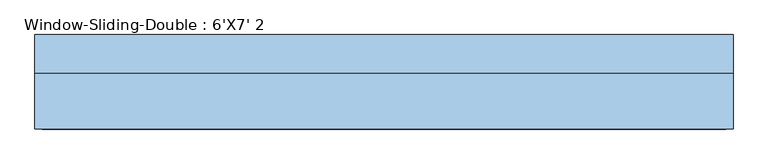
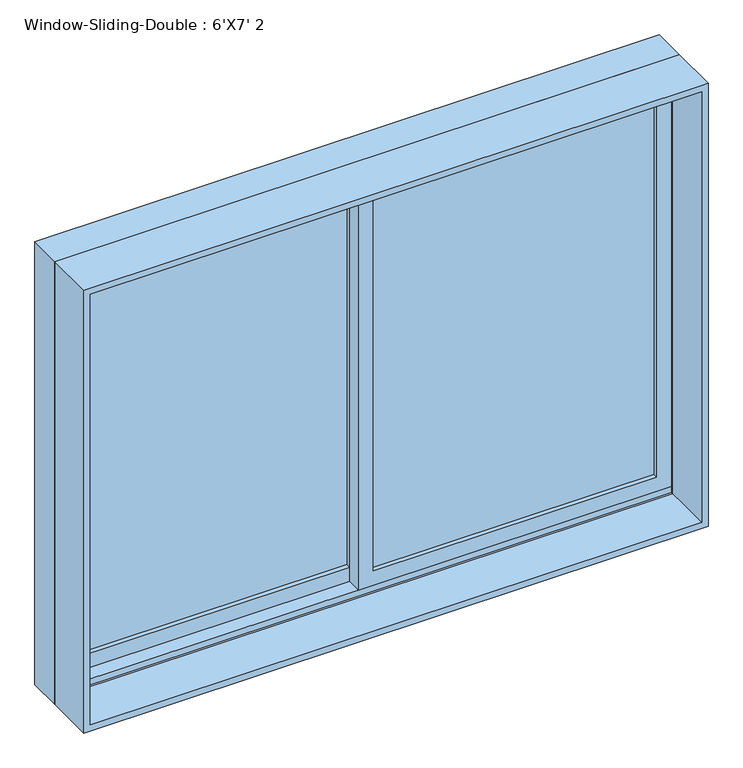
"""IFC4 building model written with IfcOpenShell, lengths in millimetres: window geometry, Window-Sliding-Double : 6'X7' 2."""

from ifc_helpers import new_model, si_unit, frame, origin, place, context, project, spatial, polyline, outline, extrude, faceted_brep, source, transform, mapped, element, save


def window_sliding_double_6_x7_2_7e5eac46(model_context):
    return source(origin(), model_context, "Body", "SolidModel", [
        extrude(outline(polyline([(952.5, 895.35), (2266.95, 895.35), (2266.95, -22.225), (952.5, -22.225), (952.5, 895.35)]), holes=[polyline([(996.95, 22.225), (2222.5, 22.225), (2222.5, 850.9), (996.95, 850.9), (996.95, 22.225)])]), frame((0.0, 34.29, 0.0), z_axis=(0.0, 1.0, 0.0), x_axis=(0.0, 0.0, 1.0)), (0.0, 0.0, 1.0), 44.45),
        extrude(outline(polyline([(933.45, -895.35), (933.45, 22.225), (2266.95, 22.225), (2266.95, -895.35), (933.45, -895.35)]), holes=[polyline([(2222.5, -22.225), (996.95, -22.225), (996.95, -850.9), (2222.5, -850.9), (2222.5, -22.225)])]), frame((0.0, 78.74, 0.0), z_axis=(0.0, 1.0, 0.0), x_axis=(0.0, 0.0, 1.0)), (0.0, 0.0, 1.0), 44.45),
        extrude(outline(polyline([(-22.225, 110.49), (-22.225, 104.14), (-850.9, 104.14), (-850.9, 110.49), (-22.225, 110.49)])), frame((0.0, 0.0, 996.95), z_axis=(0.0, 0.0, 1.0), x_axis=(1.0, 0.0, 0.0)), (0.0, 0.0, 1.0), 1225.55),
        extrude(outline(polyline([(-22.225, 97.79), (-22.225, 91.44), (-850.9, 91.44), (-850.9, 97.79), (-22.225, 97.79)])), frame((0.0, 0.0, 996.95), z_axis=(0.0, 0.0, 1.0), x_axis=(1.0, 0.0, 0.0)), (0.0, 0.0, 1.0), 1225.55),
        extrude(outline(polyline([(850.9, 66.04), (850.9, 59.69), (22.225, 59.69), (22.225, 66.04), (850.9, 66.04)])), frame((0.0, 0.0, 996.95), z_axis=(0.0, 0.0, 1.0), x_axis=(1.0, 0.0, 0.0)), (0.0, 0.0, 1.0), 1225.55),
        extrude(outline(polyline([(850.9, 53.34), (850.9, 46.99), (22.225, 46.99), (22.225, 53.34), (850.9, 53.34)])), frame((0.0, 0.0, 996.95), z_axis=(0.0, 0.0, 1.0), x_axis=(1.0, 0.0, 0.0)), (0.0, 0.0, 1.0), 1225.55),
        extrude(outline(polyline([(2286.0, -914.4), (914.4, -914.4), (914.4, 914.4), (2286.0, 914.4), (2286.0, -914.4)]), holes=[polyline([(2266.95, 895.35), (933.45, 895.35), (933.45, -895.35), (2266.95, -895.35), (2266.95, 895.35)])]), frame((0.0, -118.11, 0.0), z_axis=(0.0, 1.0, 0.0), x_axis=(0.0, 0.0, 1.0)), (0.0, 0.0, 1.0), 146.05),
        faceted_brep([(-914.4, 27.94, 914.4), (-914.4, 129.54, 914.4), (914.4, 129.54, 914.4), (914.4, 27.94, 914.4), (-873.4778905, 129.54, 2245.0778905), (-873.4778905, 123.19, 2245.0778905), (-873.4778905, 123.19, 933.45), (-873.4778905, 129.54, 933.45), (873.4778905, 123.19, 2245.0778905), (873.4778905, 123.19, 933.45), (895.35, 123.19, 933.45), (895.35, 123.19, 2266.95), (-895.35, 123.19, 2266.95), (-895.35, 123.19, 933.45), (-895.35, 27.94, 2266.95), (-895.35, 27.94, 933.45), (-895.35, 34.29, 933.45), (-895.35, 34.29, 952.5), (-895.35, 78.74, 952.5), (-895.35, 78.74, 933.45), (914.4, 27.94, 2286.0), (-914.4, 27.94, 2286.0), (895.35, 27.94, 2266.95), (895.35, 27.94, 933.45), (-914.4, 129.54, 2286.0), (914.4, 129.54, 2286.0), (873.4778905, 129.54, 933.45), (873.4778905, 129.54, 2245.0778905), (895.35, 78.74, 933.45), (895.35, 78.74, 952.5), (895.35, 34.29, 952.5), (895.35, 34.29, 933.45)], [[[0, 1, 2, 3]], [[4, 5, 6, 7]], [[5, 8, 9, 10, 11, 12, 13, 6]], [[12, 14, 15, 16, 17, 18, 19, 13]], [[0, 3, 20, 21], [22, 23, 15, 14]], [[24, 1, 0, 21]], [[2, 1, 24, 25], [4, 7, 26, 27]], [[5, 4, 27, 8]], [[12, 11, 22, 14]], [[21, 20, 25, 24]], [[8, 27, 26, 9]], [[22, 11, 10, 28, 29, 30, 31, 23]], [[20, 3, 2, 25]], [[26, 7, 6, 13, 19, 28, 10, 9]], [[28, 19, 18, 29]], [[29, 18, 17, 30]], [[30, 17, 16, 31]], [[15, 23, 31, 16]]]),
    ])


if __name__ == "__main__":
    model = new_model("IFC4")
    model_context = context("Model", 3, world=origin())
    ifc_project = project(units=[si_unit("LENGTHUNIT", "METRE", prefix="MILLI")], contexts=[model_context])
    site = spatial("IfcSite", under=ifc_project)
    building = spatial("IfcBuilding", under=site)
    placement = place(None, origin())
    window_sliding_double_6_x7_2_shape = window_sliding_double_6_x7_2_7e5eac46(model_context)
    element("IfcWindow", 1, ObjectType="Window-Sliding-Double : 6'X7' 2", at=placement, inside=building, context=model_context, shape_type="MappedRepresentation", body=[
        mapped(window_sliding_double_6_x7_2_shape, transform((0.0, 0.0, 0.0), x_axis=(1.0, 0.0, 0.0), y_axis=(0.0, 1.0, 0.0), z_axis=(0.0, 0.0, 1.0))),
    ])
    save(model, "model.ifc")

# Revit data of these elements
# Type "Window-Sliding-Double : 6'X7' 2"
#   Type Mark = "23"
#   Fire Rating = "0.5h"
#   Assembly Code = "B2020100"
#   Analytic Construction = "Double glazing - domestic"
#   Window Inset [instance default] = 0' - 0"
#   Wall Thickness [instance default] = 0' - 6"
#   Visual Light Transmittance = 0.81
#   Thermal Resistance (R) = 1.8146 (h·ft²·°F)/BTU
#   Solar Heat Gain Coefficient = 0.76
#   Muntin Width = 2' - 8 5/8"
#   Muntin Height = 4' - 0 1/4"
#   Interior Wall Closure [instance default] = 0' - 2 3/4"
#   Heat Transfer Coefficient (U) = 0.5511 BTU/(h·ft²·°F)
#   Frame Extension [instance default] = 0' - 0 1/4"
#   Exterior Wall Closure [instance default] = 0' - 1 1/4"
#   Rough Width = 6' - 0 1/2"
#   Rough Height = 4' - 6 1/2"
#   Height = 4' - 6"
#   Extension Jamb [instance default] = 0' - 2 3/4"
#   Default Sill Height = 3' - 0"
#   Width = 6' - 0"
#   Interior Trim Visibility [instance default] = yes
#   Indicator Visibility [instance default] = yes
#   Exterior Trim Visibility [instance default] = yes
#   Muntin Visibility = yes
#   Extension Jamb Visibility [instance default] = yes
#   Muntin Pattern = Muntin Pattern_2x2 : Muntin Pattern_2x2
#   Interior Trim Material = Wood - Stained
#   Interior Trim = Trim-Window-Interior-Flat : Picture Frame
#   Interior Frame Material = Wood - Stained
#   Glass Panel Material = Glass
#   Exterior Trim Material = Clad - White
#   Exterior Trim = Trim-Window-Exterior-Flat : with Sill
#   Exterior Frame Material = Clad - White
#   Wall Closure = (empty or 0)
# Element 1 (IfcWindow, "Window-Sliding-Double : 6'X7' 2")
#   Wall Thickness = 0' - 9"
#   Extension Jamb = 0' - 5 3/4"
#   Materials on its faces: "Wood - Stained", "Glass", "Clad - White"
# Materials
#   "Wood - Stained": class "Wood", colour RGB 224 178 126, transparency 0, Cost = 0
#   "Glass": class "Glass", colour RGB 0 128 192, transparency 0.75, Description = "Soda Lime Glass", Cost = 0
#   "Clad - White": class "Wood", colour RGB 242 242 238, transparency 0, Cost = 0
